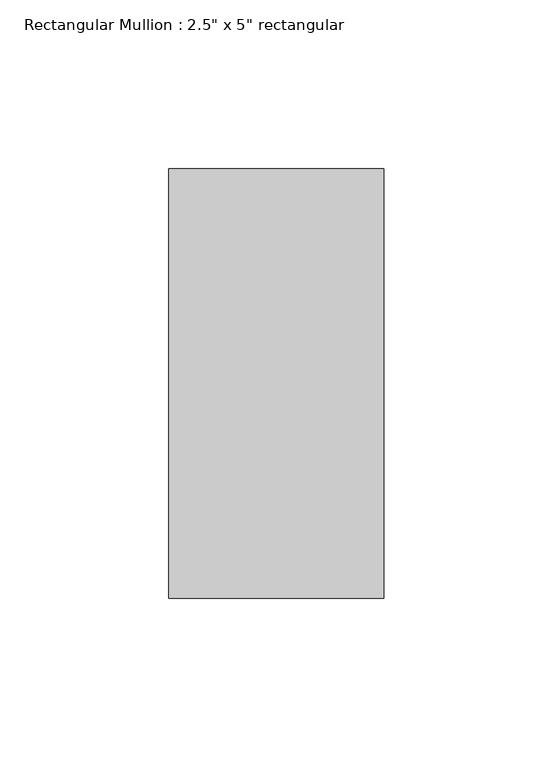
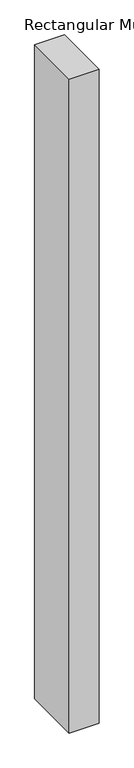
"""IFC4 building model written with IfcOpenShell, lengths in millimetres: member geometry."""

from ifc_helpers import new_model, si_unit, frame, origin, place, context, project, spatial, polyline, outline, extrude, source, transform, mapped, element, save


def member_79ea1398(model_context):
    return source(origin(), model_context, "Body", "SweptSolid", [
        extrude(outline(polyline([(31.75, 63.5), (31.75, -63.5), (-31.75, -63.5), (-31.75, 63.5), (31.75, 63.5)])), frame((0.0, 0.0, -1471.9817095), z_axis=(0.0, 0.0, 1.0), x_axis=(1.0, 0.0, 0.0)), (0.0, 0.0, 1.0), 1471.9817095),
    ])


if __name__ == "__main__":
    model = new_model("IFC4")
    model_context = context("Model", 3, world=origin())
    ifc_project = project(units=[si_unit("LENGTHUNIT", "METRE", prefix="MILLI")], contexts=[model_context])
    site = spatial("IfcSite", under=ifc_project)
    building = spatial("IfcBuilding", under=site)
    placement = place(None, origin())
    member_shape = member_79ea1398(model_context)
    element("IfcMember", 1, ObjectType="Rectangular Mullion : 2.5\" x 5\" rectangular", at=placement, inside=building, context=model_context, shape_type="MappedRepresentation", body=[
        mapped(member_shape, transform((0.0, 0.0, 0.0), x_axis=(1.0, 0.0, 0.0), y_axis=(0.0, 1.0, 0.0), z_axis=(0.0, 0.0, 1.0))),
    ])
    save(model, "model.ifc")

# Revit data of these elements
# Type "Rectangular Mullion : 2.5\" x 5\" rectangular"
#   built-in parameter 1007304 = 0.416667 (stored number, unit not read)
#   built-in parameter 1007301 = 0.104167 (stored number, unit not read)
#   built-in parameter 1007300 = 0.104167 (stored number, unit not read)
# Element 1 (IfcMember, "Rectangular Mullion : 2.5\" x 5\" rectangular")
#   Materials on its faces: "Aluminum"
# Materials
#   "Aluminum": class "Metal", colour RGB 247 247 247, transparency 0, Description = "Aluminum 6061", Cost = 0
